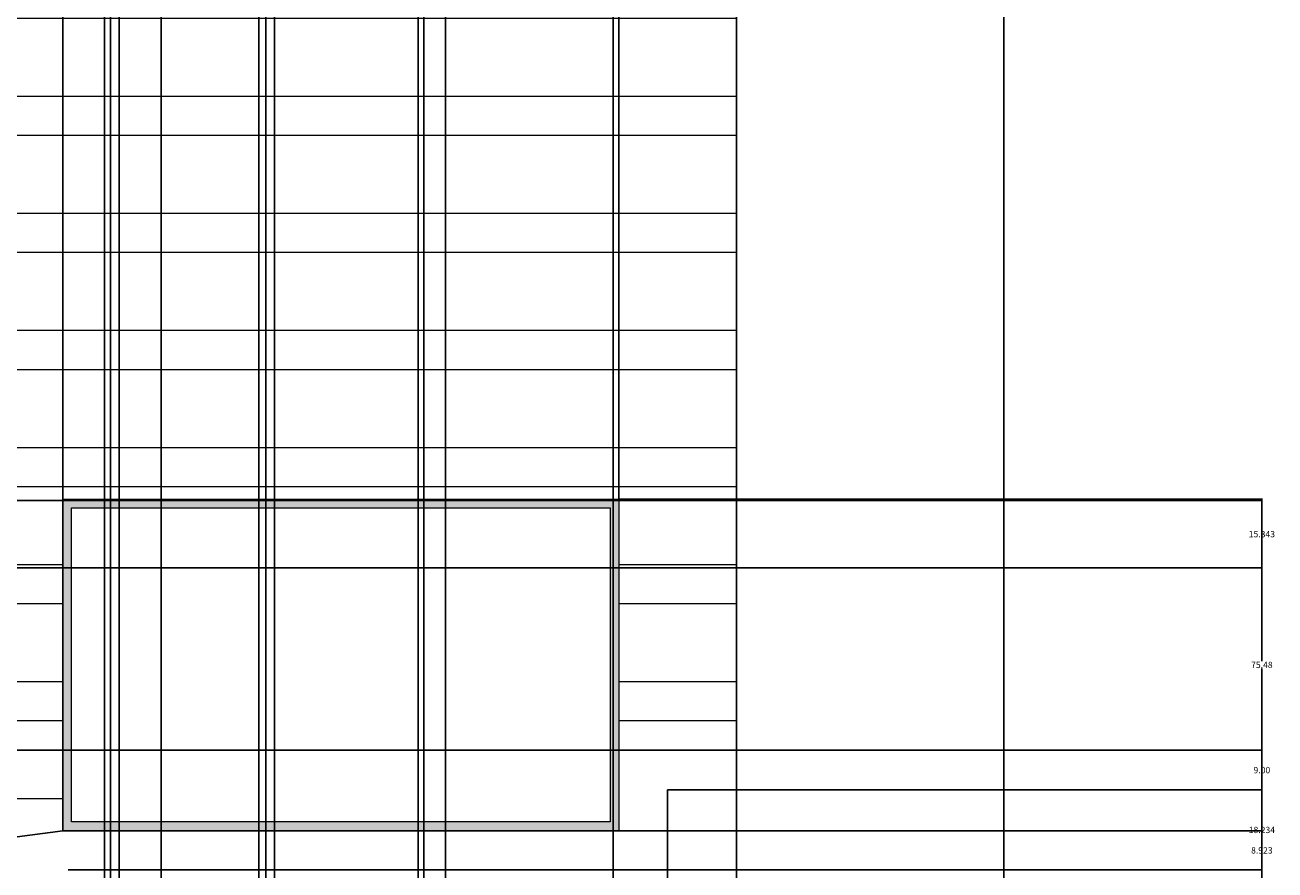
# Model space of a CAD drawing. Units: inches. Extents: x 241 to 943, y 109 to 1396.
# Tile 5 of 34: x 659 to 943, y 206 to 398. Entities that reach past the tile are written whole.
import ezdxf

# ---------------------------------------------------------------- set-up
doc = ezdxf.new("R2010")
doc.units = ezdxf.units.IN
doc.header["$MEASUREMENT"] = 0
for name, color, linetype, lineweight in [('A-ANNO-DIMS', 2, 'Continuous', 18), ('A-ELEV', 7, 'Continuous', 25), ('A-ELEV-SHAD', 9, 'Continuous', 13), ('A-GLAZ', 4, 'Continuous', 18), ('A-GLAZ-PATT', 18, 'Continuous', 13), ('A-WALL-PATT', 8, 'Continuous', 13)]:
    doc.layers.add(name, color=color, linetype=linetype, lineweight=lineweight)
doc.styles.get("Standard").update_dxf_attribs({"font": 'arial.ttf'})
doc.dimstyles.get("Standard").update_dxf_attribs({"dimtxt": 1.4375, "dimasz": 0.18, "dimexe": 0.18, "dimexo": 0.0625, "dimgap": 0.09, "dimtad": 0, "dimtih": 1, "dimtoh": 1, "dimdec": 4, "dimzin": 0, "dimdsep": 46, "dimlunit": 4, "dimtxsty": 'Standard', "dimcen": 0.09, "dimadec": 0, "dimazin": 0, "dimtfac": 1, "dimtdec": 4, "dimtofl": 0, "dimtmove": 0, "dimatfit": 3, "dimfxl": 1, "dimtolj": 1, "dimtzin": 0, "dimarcsym": 0})

# ---------------------------------------------------------------- blocks, each defined once
blk = doc.blocks.new('*D4')
at = {"layer": 'A-ANNO-DIMS', "color": 0, "lineweight": -2, "transparency": 16777216}
for p, q in [((820.84, 232.77), (820.84, 109.81)), ((377.04, 177.64), (377.04, 109.81)), ((377.22, 109.99), (596.39, 109.99)), ((820.66, 109.99), (601.48, 109.99))]:
    blk.add_line(p, q, dxfattribs=at)
at = {"layer": 'A-ANNO-DIMS', "color": 0, "transparency": 16777216}
for points in [[(377.22, 110.02), (377.22, 109.96), (377.04, 109.99)], [(820.66, 110.02), (820.66, 109.96), (820.84, 109.99)]]:
    blk.add_solid(points, dxfattribs=at)
at = {"layer": 'Defpoints', "color": 0, "transparency": 16777216}
for p in [(820.84, 232.83), (377.04, 177.7), (820.84, 109.99)]:
    blk.add_point(p, dxfattribs=at)
at = {"layer": 'A-ANNO-DIMS', "color": 0, "transparency": 16777216, "insert": (598.94, 109.99), "char_height": 1.438, "attachment_point": 5}
blk.add_mtext('\\A1;443.8', dxfattribs=at)
blk = doc.blocks.new('*D6')
at = {"layer": 'A-ANNO-DIMS', "color": 0, "lineweight": -2, "transparency": 16777216}
for p, q in [((820.84, 232.89), (820.84, 1395.05)), ((821.02, 1394.87), (848.73, 1394.87)), ((881.49, 1394.87), (853.77, 1394.87)), ((881.67, 232.89), (881.67, 1395.05))]:
    blk.add_line(p, q, dxfattribs=at)
at = {"layer": 'A-ANNO-DIMS', "color": 0, "transparency": 16777216}
for points in [[(821.02, 1394.9), (821.02, 1394.84), (820.84, 1394.87)], [(881.49, 1394.9), (881.49, 1394.84), (881.67, 1394.87)]]:
    blk.add_solid(points, dxfattribs=at)
at = {"layer": 'Defpoints', "color": 0, "transparency": 16777216}
for p in [(881.67, 1394.87), (820.84, 232.83), (881.67, 232.83)]:
    blk.add_point(p, dxfattribs=at)
at = {"layer": 'A-ANNO-DIMS', "color": 0, "transparency": 16777216, "insert": (851.25, 1394.87), "char_height": 1.438, "attachment_point": 5}
blk.add_mtext('\\A1;60.83', dxfattribs=at)
blk = doc.blocks.new('*D13')
at = {"layer": 'A-ANNO-DIMS', "color": 0, "lineweight": -2, "transparency": 16777216}
for p, q in [((650.91, 384.24), (650.91, 1395.05)), ((651.09, 1394.87), (656.14, 1394.87)), ((667.21, 1394.87), (662.16, 1394.87)), ((667.39, 290.06), (667.39, 1395.05))]:
    blk.add_line(p, q, dxfattribs=at)
at = {"layer": 'A-ANNO-DIMS', "color": 0, "transparency": 16777216}
for points in [[(651.09, 1394.9), (651.09, 1394.84), (650.91, 1394.87)], [(667.21, 1394.9), (667.21, 1394.84), (667.39, 1394.87)]]:
    blk.add_solid(points, dxfattribs=at)
at = {"layer": 'Defpoints', "color": 0, "transparency": 16777216}
for p in [(667.39, 1394.87), (650.91, 384.18), (667.39, 290)]:
    blk.add_point(p, dxfattribs=at)
at = {"layer": 'A-ANNO-DIMS', "color": 0, "transparency": 16777216, "insert": (659.15, 1394.87), "char_height": 1.438, "attachment_point": 5}
blk.add_mtext('\\A1;16.486', dxfattribs=at)
blk = doc.blocks.new('*D14')
at = {"layer": 'A-ANNO-DIMS', "color": 0, "lineweight": -2, "transparency": 16777216}
for p, q in [((667.39, 290.06), (667.39, 1395.05)), ((667.57, 1394.87), (727.7, 1394.87)), ((793.85, 1394.87), (733.72, 1394.87)), ((794.03, 290.06), (794.03, 1395.05))]:
    blk.add_line(p, q, dxfattribs=at)
at = {"layer": 'A-ANNO-DIMS', "color": 0, "transparency": 16777216}
for points in [[(667.57, 1394.9), (667.57, 1394.84), (667.39, 1394.87)], [(793.85, 1394.9), (793.85, 1394.84), (794.03, 1394.87)]]:
    blk.add_solid(points, dxfattribs=at)
at = {"layer": 'Defpoints', "color": 0, "transparency": 16777216}
for p in [(794.03, 1394.87), (667.39, 290), (794.03, 290)]:
    blk.add_point(p, dxfattribs=at)
at = {"layer": 'A-ANNO-DIMS', "color": 0, "transparency": 16777216, "insert": (730.71, 1394.87), "char_height": 1.438, "attachment_point": 5}
blk.add_mtext('\\A1;126.63', dxfattribs=at)
blk = doc.blocks.new('*D15')
at = {"layer": 'A-ANNO-DIMS', "color": 0, "lineweight": -2, "transparency": 16777216}
for p, q in [((794.03, 290.06), (794.03, 1395.05)), ((794.21, 1394.87), (805.04, 1394.87)), ((820.66, 1394.87), (809.82, 1394.87)), ((820.84, 232.89), (820.84, 1395.05))]:
    blk.add_line(p, q, dxfattribs=at)
at = {"layer": 'A-ANNO-DIMS', "color": 0, "transparency": 16777216}
for points in [[(794.21, 1394.9), (794.21, 1394.84), (794.03, 1394.87)], [(820.66, 1394.9), (820.66, 1394.84), (820.84, 1394.87)]]:
    blk.add_solid(points, dxfattribs=at)
at = {"layer": 'Defpoints', "color": 0, "transparency": 16777216}
for p in [(820.84, 1394.87), (794.03, 290), (820.84, 232.83)]:
    blk.add_point(p, dxfattribs=at)
at = {"layer": 'A-ANNO-DIMS', "color": 0, "transparency": 16777216, "insert": (807.43, 1394.87), "char_height": 1.438, "attachment_point": 5}
blk.add_mtext('\\A1;26.81', dxfattribs=at)
blk = doc.blocks.new('*D29')
at = {"layer": 'A-ANNO-DIMS', "color": 0, "lineweight": -2, "transparency": 16777216}
for p, q in [((462.17, 289.69), (940.6, 289.69)), ((940.42, 289.51), (940.42, 282.85)), ((940.42, 274.53), (940.42, 281.2)), ((462.17, 274.35), (940.6, 274.35))]:
    blk.add_line(p, q, dxfattribs=at)
at = {"layer": 'A-ANNO-DIMS', "color": 0, "transparency": 16777216}
for points in [[(940.39, 289.51), (940.45, 289.51), (940.42, 289.69)], [(940.39, 274.53), (940.45, 274.53), (940.42, 274.35)]]:
    blk.add_solid(points, dxfattribs=at)
at = {"layer": 'Defpoints', "color": 0, "transparency": 16777216}
for p in [(462.11, 289.69), (940.42, 289.69), (462.11, 274.35)]:
    blk.add_point(p, dxfattribs=at)
at = {"layer": 'A-ANNO-DIMS', "color": 0, "transparency": 16777216, "insert": (940.42, 282.02), "char_height": 1.438, "attachment_point": 5}
blk.add_mtext('\\A1;15.343', dxfattribs=at)
blk = doc.blocks.new('*D41')
at = {"layer": 'A-ANNO-DIMS', "color": 0, "lineweight": -2, "transparency": 16777216}
for p, q in [((820.77, 400.83), (244.31, 400.83)), ((244.49, 400.65), (244.49, 317.65)), ((244.49, 233.01), (244.49, 316.01)), ((820.77, 232.83), (244.31, 232.83))]:
    blk.add_line(p, q, dxfattribs=at)
at = {"layer": 'A-ANNO-DIMS', "color": 0, "transparency": 16777216}
for points in [[(244.46, 400.65), (244.52, 400.65), (244.49, 400.83)], [(244.46, 233.01), (244.52, 233.01), (244.49, 232.83)]]:
    blk.add_solid(points, dxfattribs=at)
at = {"layer": 'Defpoints', "color": 0, "transparency": 16777216}
for p in [(244.49, 400.83), (820.84, 400.83), (820.84, 232.83)]:
    blk.add_point(p, dxfattribs=at)
at = {"layer": 'A-ANNO-DIMS', "color": 0, "transparency": 16777216, "insert": (244.49, 316.83), "char_height": 1.438, "attachment_point": 5}
blk.add_mtext('\\A1;168', dxfattribs=at)
blk = doc.blocks.new('*D44')
at = {"layer": 'A-ANNO-DIMS', "color": 0, "lineweight": -2, "transparency": 16777216}
for p, q in [((794.09, 290), (940.6, 290)), ((940.42, 289.82), (940.42, 253.08)), ((940.42, 214.7), (940.42, 251.43)), ((794.09, 214.52), (940.6, 214.52))]:
    blk.add_line(p, q, dxfattribs=at)
at = {"layer": 'A-ANNO-DIMS', "color": 0, "transparency": 16777216}
for points in [[(940.39, 289.82), (940.45, 289.82), (940.42, 290)], [(940.39, 214.7), (940.45, 214.7), (940.42, 214.52)]]:
    blk.add_solid(points, dxfattribs=at)
at = {"layer": 'Defpoints', "color": 0, "transparency": 16777216}
for p in [(794.03, 290), (940.42, 290), (794.03, 214.52)]:
    blk.add_point(p, dxfattribs=at)
at = {"layer": 'A-ANNO-DIMS', "color": 0, "transparency": 16777216, "insert": (940.42, 252.26), "char_height": 1.438, "attachment_point": 5}
blk.add_mtext('\\A1;75.48', dxfattribs=at)
blk = doc.blocks.new('*D75')
at = {"layer": 'A-ANNO-DIMS', "color": 0, "lineweight": -2, "transparency": 16777216}
for p, q in [((667.46, 214.52), (940.6, 214.52)), ((940.42, 214.34), (940.42, 196.93)), ((940.42, 177.88), (940.42, 195.28)), ((377.1, 177.7), (940.6, 177.7))]:
    blk.add_line(p, q, dxfattribs=at)
at = {"layer": 'A-ANNO-DIMS', "color": 0, "transparency": 16777216}
for points in [[(940.39, 214.34), (940.45, 214.34), (940.42, 214.52)], [(940.39, 177.88), (940.45, 177.88), (940.42, 177.7)]]:
    blk.add_solid(points, dxfattribs=at)
at = {"layer": 'Defpoints', "color": 0, "transparency": 16777216}
for p in [(667.39, 214.52), (940.42, 214.52), (377.04, 177.7)]:
    blk.add_point(p, dxfattribs=at)
at = {"layer": 'A-ANNO-DIMS', "color": 0, "transparency": 16777216, "insert": (940.42, 196.11), "char_height": 1.438, "attachment_point": 5}
blk.add_mtext('\\A1;36.82', dxfattribs=at)
blk = doc.blocks.new('*D76')
at = {"layer": 'A-ANNO-DIMS', "color": 0, "lineweight": -2, "transparency": 16777216}
for p, q in [((805.12, 223.83), (940.6, 223.83)), ((940.42, 223.65), (940.42, 215.54)), ((940.42, 205.78), (940.42, 213.89)), ((805.12, 205.6), (940.6, 205.6))]:
    blk.add_line(p, q, dxfattribs=at)
at = {"layer": 'A-ANNO-DIMS', "color": 0, "transparency": 16777216}
for points in [[(940.39, 223.65), (940.45, 223.65), (940.42, 223.83)], [(940.39, 205.78), (940.45, 205.78), (940.42, 205.6)]]:
    blk.add_solid(points, dxfattribs=at)
at = {"layer": 'Defpoints', "color": 0, "transparency": 16777216}
for p in [(805.06, 223.83), (940.42, 223.83), (805.06, 205.6)]:
    blk.add_point(p, dxfattribs=at)
at = {"layer": 'A-ANNO-DIMS', "color": 0, "transparency": 16777216, "insert": (940.42, 214.71), "char_height": 1.438, "attachment_point": 5}
blk.add_mtext('\\A1;18.234', dxfattribs=at)
blk = doc.blocks.new('*D77')
at = {"layer": 'A-ANNO-DIMS', "color": 0, "lineweight": -2, "transparency": 16777216}
for p, q in [((805.06, 223.77), (805.06, 109.81)), ((881.67, 223.77), (881.67, 109.81)), ((805.24, 109.99), (840.99, 109.99)), ((881.49, 109.99), (845.73, 109.99))]:
    blk.add_line(p, q, dxfattribs=at)
at = {"layer": 'A-ANNO-DIMS', "color": 0, "transparency": 16777216}
for points in [[(805.24, 110.02), (805.24, 109.96), (805.06, 109.99)], [(881.49, 110.02), (881.49, 109.96), (881.67, 109.99)]]:
    blk.add_solid(points, dxfattribs=at)
at = {"layer": 'Defpoints', "color": 0, "transparency": 16777216}
for p in [(805.06, 223.83), (881.67, 223.83), (881.67, 109.99)]:
    blk.add_point(p, dxfattribs=at)
at = {"layer": 'A-ANNO-DIMS', "color": 0, "transparency": 16777216, "insert": (843.36, 109.99), "char_height": 1.438, "attachment_point": 5}
blk.add_mtext('\\A1;76.61', dxfattribs=at)
blk = doc.blocks.new('*D78')
at = {"layer": 'A-ANNO-DIMS', "color": 0, "lineweight": -2, "transparency": 16777216}
for p, q in [((881.73, 232.83), (940.6, 232.83)), ((940.42, 232.65), (940.42, 229.15)), ((940.42, 224.01), (940.42, 227.51)), ((881.73, 223.83), (940.6, 223.83))]:
    blk.add_line(p, q, dxfattribs=at)
at = {"layer": 'A-ANNO-DIMS', "color": 0, "transparency": 16777216}
for points in [[(940.39, 232.65), (940.45, 232.65), (940.42, 232.83)], [(940.39, 224.01), (940.45, 224.01), (940.42, 223.83)]]:
    blk.add_solid(points, dxfattribs=at)
at = {"layer": 'Defpoints', "color": 0, "transparency": 16777216}
for p in [(881.67, 232.83), (940.42, 232.83), (881.67, 223.83)]:
    blk.add_point(p, dxfattribs=at)
at = {"layer": 'A-ANNO-DIMS', "color": 0, "transparency": 16777216, "insert": (940.42, 228.33), "char_height": 1.438, "attachment_point": 5}
blk.add_mtext('\\A1;9.00', dxfattribs=at)
blk = doc.blocks.new('*D97')
at = {"layer": 'A-ANNO-DIMS', "color": 0, "lineweight": -2, "transparency": 16777216}
for p, q in [((881.67, 223.77), (881.67, 109.81)), ((303.24, 168.68), (303.24, 109.81)), ((303.42, 109.99), (589.38, 109.99)), ((881.49, 109.99), (595.53, 109.99))]:
    blk.add_line(p, q, dxfattribs=at)
at = {"layer": 'A-ANNO-DIMS', "color": 0, "transparency": 16777216}
for points in [[(303.42, 110.02), (303.42, 109.96), (303.24, 109.99)], [(881.49, 110.02), (881.49, 109.96), (881.67, 109.99)]]:
    blk.add_solid(points, dxfattribs=at)
at = {"layer": 'Defpoints', "color": 0, "transparency": 16777216}
for p in [(881.67, 223.83), (303.24, 168.74), (881.67, 109.99)]:
    blk.add_point(p, dxfattribs=at)
at = {"layer": 'A-ANNO-DIMS', "color": 0, "transparency": 16777216, "insert": (592.45, 109.99), "char_height": 1.438, "attachment_point": 5}
blk.add_mtext('\\A1;578.43', dxfattribs=at)
blk = doc.blocks.new('*D99')
at = {"layer": 'A-ANNO-DIMS', "color": 0, "lineweight": -2, "transparency": 16777216}
for p, q in [((417.09, 181.71), (417.09, 1395.05)), ((417.27, 1394.87), (539.16, 1394.87)), ((667.21, 1394.87), (545.33, 1394.87)), ((667.39, 214.58), (667.39, 1395.05))]:
    blk.add_line(p, q, dxfattribs=at)
at = {"layer": 'A-ANNO-DIMS', "color": 0, "transparency": 16777216}
for points in [[(417.27, 1394.9), (417.27, 1394.84), (417.09, 1394.87)], [(667.21, 1394.9), (667.21, 1394.84), (667.39, 1394.87)]]:
    blk.add_solid(points, dxfattribs=at)
at = {"layer": 'Defpoints', "color": 0, "transparency": 16777216}
for p in [(667.39, 1394.87), (667.39, 214.52), (417.09, 181.65)]:
    blk.add_point(p, dxfattribs=at)
at = {"layer": 'A-ANNO-DIMS', "color": 0, "transparency": 16777216, "insert": (542.24, 1394.87), "char_height": 1.438, "attachment_point": 5}
blk.add_mtext('\\A1;250.30', dxfattribs=at)
blk = doc.blocks.new('*D100')
at = {"layer": 'A-ANNO-DIMS', "color": 0, "lineweight": -2, "transparency": 16777216}
for p, q in [((667.46, 214.52), (940.6, 214.52)), ((940.42, 214.34), (940.42, 210.88)), ((940.42, 205.78), (940.42, 209.23)), ((668.63, 205.6), (940.6, 205.6))]:
    blk.add_line(p, q, dxfattribs=at)
at = {"layer": 'A-ANNO-DIMS', "color": 0, "transparency": 16777216}
for points in [[(940.39, 214.34), (940.45, 214.34), (940.42, 214.52)], [(940.39, 205.78), (940.45, 205.78), (940.42, 205.6)]]:
    blk.add_solid(points, dxfattribs=at)
at = {"layer": 'Defpoints', "color": 0, "transparency": 16777216}
for p in [(667.39, 214.52), (940.42, 214.52), (668.57, 205.6)]:
    blk.add_point(p, dxfattribs=at)
at = {"layer": 'A-ANNO-DIMS', "color": 0, "transparency": 16777216, "insert": (940.42, 210.06), "char_height": 1.438, "attachment_point": 5}
blk.add_mtext('\\A1;8.923', dxfattribs=at)
blk = doc.blocks.new('*D120')
at = {"layer": 'A-ANNO-DIMS', "color": 0, "lineweight": -2, "transparency": 16777216}
for p, q in [((642.92, 734.79), (642.92, 109.81)), ((678.27, 734.79), (678.27, 109.81)), ((643.1, 109.99), (658.07, 109.99)), ((678.09, 109.99), (663.11, 109.99))]:
    blk.add_line(p, q, dxfattribs=at)
at = {"layer": 'A-ANNO-DIMS', "color": 0, "transparency": 16777216}
for points in [[(643.1, 110.02), (643.1, 109.96), (642.92, 109.99)], [(678.09, 110.02), (678.09, 109.96), (678.27, 109.99)]]:
    blk.add_solid(points, dxfattribs=at)
at = {"layer": 'Defpoints', "color": 0, "transparency": 16777216}
for p in [(642.92, 734.85), (678.27, 734.85), (678.27, 109.99)]:
    blk.add_point(p, dxfattribs=at)
at = {"layer": 'A-ANNO-DIMS', "color": 0, "transparency": 16777216, "insert": (660.59, 109.99), "char_height": 1.438, "attachment_point": 5}
blk.add_mtext('\\A1;35.35', dxfattribs=at)
blk = doc.blocks.new('*D121')
at = {"layer": 'A-ANNO-DIMS', "color": 0, "lineweight": -2, "transparency": 16777216}
for p, q in [((680.27, 736.86), (680.27, 109.81)), ((713.62, 736.86), (713.62, 109.81)), ((680.45, 109.99), (693.87, 109.99)), ((713.44, 109.99), (700.02, 109.99))]:
    blk.add_line(p, q, dxfattribs=at)
at = {"layer": 'A-ANNO-DIMS', "color": 0, "transparency": 16777216}
for points in [[(680.45, 110.02), (680.45, 109.96), (680.27, 109.99)], [(713.44, 110.02), (713.44, 109.96), (713.62, 109.99)]]:
    blk.add_solid(points, dxfattribs=at)
at = {"layer": 'Defpoints', "color": 0, "transparency": 16777216}
for p in [(680.27, 736.92), (713.62, 736.92), (713.62, 109.99)]:
    blk.add_point(p, dxfattribs=at)
at = {"layer": 'A-ANNO-DIMS', "color": 0, "transparency": 16777216, "insert": (696.95, 109.99), "char_height": 1.438, "attachment_point": 5}
blk.add_mtext('\\A1;33.356', dxfattribs=at)
blk = doc.blocks.new('*D122')
at = {"layer": 'A-ANNO-DIMS', "color": 0, "lineweight": -2, "transparency": 16777216}
for p, q in [((715.62, 734.79), (715.62, 109.81)), ((754.54, 734.79), (754.54, 109.81)), ((715.8, 109.99), (732.7, 109.99)), ((754.36, 109.99), (737.46, 109.99))]:
    blk.add_line(p, q, dxfattribs=at)
at = {"layer": 'A-ANNO-DIMS', "color": 0, "transparency": 16777216}
for points in [[(715.8, 110.02), (715.8, 109.96), (715.62, 109.99)], [(754.36, 110.02), (754.36, 109.96), (754.54, 109.99)]]:
    blk.add_solid(points, dxfattribs=at)
at = {"layer": 'Defpoints', "color": 0, "transparency": 16777216}
for p in [(715.62, 734.85), (754.54, 734.85), (754.54, 109.99)]:
    blk.add_point(p, dxfattribs=at)
at = {"layer": 'A-ANNO-DIMS', "color": 0, "transparency": 16777216, "insert": (735.08, 109.99), "char_height": 1.438, "attachment_point": 5}
blk.add_mtext('\\A1;38.91', dxfattribs=at)
blk = doc.blocks.new('*D123')
at = {"layer": 'A-ANNO-DIMS', "color": 0, "lineweight": -2, "transparency": 16777216}
for p, q in [((754.54, 734.79), (754.54, 109.81)), ((792.69, 734.79), (792.69, 109.81)), ((754.72, 109.99), (771.09, 109.99)), ((792.51, 109.99), (776.13, 109.99))]:
    blk.add_line(p, q, dxfattribs=at)
at = {"layer": 'A-ANNO-DIMS', "color": 0, "transparency": 16777216}
for points in [[(754.72, 110.02), (754.72, 109.96), (754.54, 109.99)], [(792.51, 110.02), (792.51, 109.96), (792.69, 109.99)]]:
    blk.add_solid(points, dxfattribs=at)
at = {"layer": 'Defpoints', "color": 0, "transparency": 16777216}
for p in [(754.54, 734.85), (792.69, 734.85), (792.69, 109.99)]:
    blk.add_point(p, dxfattribs=at)
at = {"layer": 'A-ANNO-DIMS', "color": 0, "transparency": 16777216, "insert": (773.61, 109.99), "char_height": 1.438, "attachment_point": 5}
blk.add_mtext('\\A1;38.15', dxfattribs=at)
blk = doc.blocks.new('*D132')
at = {"layer": 'A-ANNO-DIMS', "color": 0, "lineweight": -2, "transparency": 16777216}
for p, q in [((617.76, 626.34), (617.76, 109.81)), ((676.87, 628.34), (676.87, 109.81)), ((617.94, 109.99), (644.94, 109.99)), ((676.69, 109.99), (649.69, 109.99))]:
    blk.add_line(p, q, dxfattribs=at)
at = {"layer": 'A-ANNO-DIMS', "color": 0, "transparency": 16777216}
for points in [[(617.94, 110.02), (617.94, 109.96), (617.76, 109.99)], [(676.69, 110.02), (676.69, 109.96), (676.87, 109.99)]]:
    blk.add_solid(points, dxfattribs=at)
at = {"layer": 'Defpoints', "color": 0, "transparency": 16777216}
for p in [(617.76, 626.4), (676.87, 628.4), (676.87, 109.99)]:
    blk.add_point(p, dxfattribs=at)
at = {"layer": 'A-ANNO-DIMS', "color": 0, "transparency": 16777216, "insert": (647.31, 109.99), "char_height": 1.438, "attachment_point": 5}
blk.add_mtext('\\A1;59.11', dxfattribs=at)
blk = doc.blocks.new('*D133')
at = {"layer": 'A-ANNO-DIMS', "color": 0, "lineweight": -2, "transparency": 16777216}
for p, q in [((676.87, 628.34), (676.87, 109.81)), ((712.02, 628.34), (712.02, 109.81)), ((677.05, 109.99), (691.92, 109.99)), ((711.84, 109.99), (696.96, 109.99))]:
    blk.add_line(p, q, dxfattribs=at)
at = {"layer": 'A-ANNO-DIMS', "color": 0, "transparency": 16777216}
for points in [[(677.05, 110.02), (677.05, 109.96), (676.87, 109.99)], [(711.84, 110.02), (711.84, 109.96), (712.02, 109.99)]]:
    blk.add_solid(points, dxfattribs=at)
at = {"layer": 'Defpoints', "color": 0, "transparency": 16777216}
for p in [(676.87, 628.4), (712.02, 628.4), (712.02, 109.99)]:
    blk.add_point(p, dxfattribs=at)
at = {"layer": 'A-ANNO-DIMS', "color": 0, "transparency": 16777216, "insert": (694.44, 109.99), "char_height": 1.438, "attachment_point": 5}
blk.add_mtext('\\A1;35.15', dxfattribs=at)
blk = doc.blocks.new('*D134')
at = {"layer": 'A-ANNO-DIMS', "color": 0, "lineweight": -2, "transparency": 16777216}
for p, q in [((712.02, 628.34), (712.02, 109.81)), ((749.63, 626.34), (749.63, 109.81)), ((712.2, 109.99), (727.75, 109.99)), ((749.45, 109.99), (733.9, 109.99))]:
    blk.add_line(p, q, dxfattribs=at)
at = {"layer": 'A-ANNO-DIMS', "color": 0, "transparency": 16777216}
for points in [[(712.2, 110.02), (712.2, 109.96), (712.02, 109.99)], [(749.45, 110.02), (749.45, 109.96), (749.63, 109.99)]]:
    blk.add_solid(points, dxfattribs=at)
at = {"layer": 'Defpoints', "color": 0, "transparency": 16777216}
for p in [(712.02, 628.4), (749.63, 626.4), (749.63, 109.99)]:
    blk.add_point(p, dxfattribs=at)
at = {"layer": 'A-ANNO-DIMS', "color": 0, "transparency": 16777216, "insert": (730.82, 109.99), "char_height": 1.438, "attachment_point": 5}
blk.add_mtext('\\A1;37.616', dxfattribs=at)
blk = doc.blocks.new('*D142')
at = {"layer": 'A-ANNO-DIMS', "color": 0, "lineweight": -2, "transparency": 16777216}
for p, q in [((689.79, 498.38), (689.79, 109.81)), ((651.6, 496.38), (651.6, 109.81)), ((651.78, 109.99), (668.18, 109.99)), ((689.61, 109.99), (673.21, 109.99))]:
    blk.add_line(p, q, dxfattribs=at)
at = {"layer": 'A-ANNO-DIMS', "color": 0, "transparency": 16777216}
for points in [[(651.78, 110.02), (651.78, 109.96), (651.6, 109.99)], [(689.61, 110.02), (689.61, 109.96), (689.79, 109.99)]]:
    blk.add_solid(points, dxfattribs=at)
at = {"layer": 'Defpoints', "color": 0, "transparency": 16777216}
for p in [(689.79, 498.44), (651.6, 496.44), (689.79, 109.99)]:
    blk.add_point(p, dxfattribs=at)
at = {"layer": 'A-ANNO-DIMS', "color": 0, "transparency": 16777216, "insert": (670.7, 109.99), "char_height": 1.438, "attachment_point": 5}
blk.add_mtext('\\A1;38.20', dxfattribs=at)
blk = doc.blocks.new('*D143')
at = {"layer": 'A-ANNO-DIMS', "color": 0, "lineweight": -2, "transparency": 16777216}
for p, q in [((689.79, 498.38), (689.79, 109.81)), ((748.33, 498.38), (748.33, 109.81)), ((689.97, 109.99), (716.55, 109.99)), ((748.15, 109.99), (721.58, 109.99))]:
    blk.add_line(p, q, dxfattribs=at)
at = {"layer": 'A-ANNO-DIMS', "color": 0, "transparency": 16777216}
for points in [[(689.97, 110.02), (689.97, 109.96), (689.79, 109.99)], [(748.15, 110.02), (748.15, 109.96), (748.33, 109.99)]]:
    blk.add_solid(points, dxfattribs=at)
at = {"layer": 'Defpoints', "color": 0, "transparency": 16777216}
for p in [(689.79, 498.44), (748.33, 498.44), (748.33, 109.99)]:
    blk.add_point(p, dxfattribs=at)
at = {"layer": 'A-ANNO-DIMS', "color": 0, "transparency": 16777216, "insert": (719.06, 109.99), "char_height": 1.438, "attachment_point": 5}
blk.add_mtext('\\A1;58.54', dxfattribs=at)
blk = doc.blocks.new('*D144')
at = {"layer": 'A-ANNO-DIMS', "color": 0, "lineweight": -2, "transparency": 16777216}
for p, q in [((748.33, 498.38), (748.33, 109.81)), ((792.69, 496.38), (792.69, 109.81)), ((748.51, 109.99), (767.97, 109.99)), ((792.51, 109.99), (773.06, 109.99))]:
    blk.add_line(p, q, dxfattribs=at)
at = {"layer": 'A-ANNO-DIMS', "color": 0, "transparency": 16777216}
for points in [[(748.51, 110.02), (748.51, 109.96), (748.33, 109.99)], [(792.51, 110.02), (792.51, 109.96), (792.69, 109.99)]]:
    blk.add_solid(points, dxfattribs=at)
at = {"layer": 'Defpoints', "color": 0, "transparency": 16777216}
for p in [(748.33, 498.44), (792.69, 496.44), (792.69, 109.99)]:
    blk.add_point(p, dxfattribs=at)
at = {"layer": 'A-ANNO-DIMS', "color": 0, "transparency": 16777216, "insert": (770.51, 109.99), "char_height": 1.438, "attachment_point": 5}
blk.add_mtext('\\A1;44.36', dxfattribs=at)

msp = doc.modelspace()

# ---------------------------------------------------------------- hatches: boundary and pattern name
at = {"layer": 'A-ELEV-SHAD'}
h = msp.add_hatch(color=256, dxfattribs=at)
h.dxf.hatch_style = 1
h.paths.add_polyline_path([(748.3325, 566.8295), (746.3325, 566.8295), (746.3325, 498.4395), (748.3325, 498.4395)])
h.paths.add_polyline_path([(746.3325, 524.3723), (691.794, 524.3723), (691.794, 522.3723), (746.3325, 522.3723)])
h.paths.add_polyline_path([(691.794, 566.8295), (689.794, 566.8295), (689.794, 498.4395), (691.794, 498.4395)])
h.paths.add_polyline_path([(790.691, 542.7994), (748.3325, 542.7994), (748.3325, 540.7994), (790.691, 540.7994)])
h.paths.add_polyline_path([(500.3323, 384.1784), (479.596, 384.1784), (479.596, 289.6933), (500.3323, 289.6933)])
h.paths.add_polyline_path([(481.596, 291.6933), (481.596, 382.1784), (498.3323, 382.1784), (498.3323, 291.6933)], flags=16)
h.paths.add_polyline_path([(462.1074, 384.1784), (390.895, 384.1784), (390.895, 289.6933), (462.1074, 289.6933)])
h.paths.add_polyline_path([(392.895, 291.6933), (392.895, 382.1784), (460.1074, 382.1784), (460.1074, 291.6933)], flags=16)
h.paths.add_polyline_path([(794.0275, 289.9984), (667.3935, 289.9984), (667.3935, 214.5189), (794.0275, 214.5189)])
h.paths.add_polyline_path([(792.0275, 287.9984), (792.0275, 216.5189), (669.3935, 216.5189), (669.3935, 287.9984)], flags=16)
h.paths.add_polyline_path([(508.0803, 525.3816), (506.0803, 525.3816), (506.0803, 521.3754), (452.9259, 521.3754), (452.9259, 525.3816), (450.9259, 525.3816), (450.9259, 519.3754), (508.0803, 519.3754)], flags=0)
h.paths.add_polyline_path([(508.0803, 566.8295), (450.9259, 566.8295), (450.9259, 527.3816), (452.9259, 527.3816), (452.9259, 564.8295), (506.0803, 564.8295), (506.0803, 527.3816), (508.0803, 527.3816)], flags=0)
h.paths.add_polyline_path([(537.4269, 566.8295), (534.1778, 566.8295), (534.1778, 527.3816), (537.4269, 527.3816)], flags=0)
h.paths.add_polyline_path([(537.4269, 525.3816), (534.1778, 525.3816), (534.1778, 508.9074), (537.4269, 508.9074)], flags=0)
h.paths.add_polyline_path([(565.2023, 568.8295), (424.1086, 568.8295), (424.1086, 496.4395), (565.2023, 496.4395)])
h.paths.add_polyline_path([(563.2023, 508.9074), (563.2023, 498.4395), (426.1086, 498.4395), (426.1086, 566.8295), (563.2023, 566.8295)], flags=16)
h.paths.add_polyline_path([(508.0803, 508.9074), (508.0803, 519.3754), (450.9259, 519.3754), (450.9259, 525.3816), (445.5808, 525.3816, -1), (445.5808, 527.3816), (450.9259, 527.3816), (450.9259, 566.8295), (508.0803, 566.8295), (537.4269, 566.8295), (537.4269, 508.9074)], flags=0)
h.paths.add_polyline_path([(506.0803, 521.3754), (452.9259, 521.3754), (452.9259, 564.8295), (506.0803, 564.8295)], flags=0)
at = {"layer": 'A-GLAZ-PATT'}
h = msp.add_hatch(dxfattribs=at)
h.set_pattern_fill('ANSI31', color=256, scale=34, angle=45)
h.paths.add_polyline_path([(486.3418, 786.9154), (413.1187, 786.9154), (413.1187, 761.2284), (486.3418, 761.2284)])
h.paths.add_polyline_path([(486.3418, 954.9154), (413.1187, 954.9154), (413.1187, 929.2284), (486.3418, 929.2284)])
h.paths.add_polyline_path([(462.1074, 289.6933), (390.895, 289.6933), (390.895, 277.4626), (390.895, 274.3507), (462.1074, 274.3507), (462.1074, 277.4626)])
h.paths.add_polyline_path([(500.3323, 289.6933), (479.596, 289.6933), (479.596, 274.3507), (500.3323, 274.3507)])
h.paths.add_polyline_path([(450.9259, 566.8295), (426.1086, 566.8295), (426.1086, 498.4395), (446.4348, 498.4395), (446.4348, 519.3754), (450.9259, 519.3754), (450.9259, 525.3816), (445.5808, 525.3816, -1), (445.5808, 527.3816), (450.9259, 527.3816)])
h.paths.add_polyline_path([(563.2023, 508.9074), (534.1778, 508.9074), (508.1906, 508.9074), (508.1906, 498.4395), (563.2023, 498.4395)])
h.paths.add_polyline_path([(747.6328, 700.7912), (712.0171, 700.7912), (712.0171, 628.4013), (747.6328, 628.4013)])
h.paths.add_polyline_path([(446.4348, 643.7483), (426.1086, 643.7483), (426.1086, 630.4013), (446.4348, 630.4013)])
h.paths.add_polyline_path([(564.8076, 841.5382), (553.5166, 841.5382), (508.3064, 841.5382), (508.3064, 782.5808), (564.8076, 782.5808)])
h.paths.add_polyline_path([(564.8076, 780.5808), (508.3064, 780.5808), (508.3064, 773.4916), (564.8076, 773.4916)])
h.paths.add_polyline_path([(792.691, 762.5799), (759.6248, 762.5799), (759.6248, 736.9235), (759.6248, 734.8538), (792.691, 734.8538)])
h.paths.add_polyline_path([(564.8076, 1009.5382), (553.5166, 1009.5382), (508.3064, 1009.5382), (508.3064, 950.5808), (562.3033, 950.5808, -1), (562.3033, 948.5808), (508.3064, 948.5808), (508.3064, 941.4916), (564.8076, 941.4916)])
h.paths.add_polyline_path([(486.3418, 1122.9154), (413.1187, 1122.9154), (413.1187, 1097.2284), (486.3418, 1097.2284)])
at = {"layer": 'A-WALL-PATT'}
h = msp.add_hatch(dxfattribs=at)
h.set_pattern_fill('ANSI32', color=256, scale=71, angle=135)
h.paths.add_polyline_path([(820.8374, 568.8295), (792.691, 568.8295), (792.691, 496.4395), (651.5974, 496.4395), (651.5974, 568.8295), (617.7594, 568.8295), (618.9643, 400.8295), (417.0913, 400.8295), (377.0391, 400.8295), (377.0391, 398.8538), (377.0391, 396.8782), (377.0391, 228.8782), (377.0391, 177.6977), (416.5078, 181.5724), (417.0913, 181.649), (530.2303, 196.5065), (530.2303, 384.1784), (650.907, 384.1784), (651.7861, 212.4693), (667.3935, 214.5189), (667.3935, 289.9984), (794.0275, 289.9984), (794.0275, 232.8295), (820.8374, 232.8295), (820.8374, 400.8295)])
h.paths.add_polyline_path([(500.3323, 384.1784), (500.3323, 289.6933), (500.3323, 274.3507), (479.596, 274.3507), (479.596, 289.6933), (479.596, 384.1784)], flags=16)
h.paths.add_polyline_path([(498.3323, 382.1784), (498.3323, 291.6933), (481.596, 291.6933), (481.596, 382.1784)], flags=0)
h.paths.add_polyline_path([(462.1074, 384.1784), (462.1074, 289.6933), (462.1074, 277.4626), (462.1074, 274.3507), (390.895, 274.3507), (390.895, 277.4626), (390.895, 289.6933), (390.895, 384.1784)], flags=16)
h.paths.add_polyline_path([(460.1074, 382.1784), (460.1074, 291.6933), (392.895, 291.6933), (392.895, 382.1784)], flags=0)
h.paths.add_polyline_path([(595.3136, 372.9401), (641.6196, 372.9401), (641.6196, 246.4081), (651.6121, 246.4593), (650.907, 384.1784), (530.2303, 384.1784), (530.2303, 245.8378), (595.3136, 246.1711)], flags=17)

# ---------------------------------------------------------------- linework, layer by layer
at = {"layer": 'A-ELEV'}
for p, q in [((820.8374, 400.8295), (820.8374, 232.8295)), ((820.8374, 232.8295), (794.0275, 232.8295)), ((820.8374, 232.8295), (881.5299, 232.8295)), ((881.5299, 232.8295), (881.667, 232.8295)), ((881.667, 223.8295), (881.667, 232.8295)), ((820.8374, 223.8295), (805.0568, 223.8295)), ((805.0568, 205.5955), (805.0568, 223.8295)), ((820.8374, 223.8295), (881.667, 223.8295)), ((667.3935, 214.5189), (417.0913, 181.649))]:
    msp.add_line(p, q, dxfattribs=at)
at = {"layer": 'A-GLAZ'}
for p, q in [((794.0275, 232.8295), (794.0275, 214.5189)), ((704.8945, 214.5189), (667.3935, 214.5189)), ((794.0275, 214.5189), (704.8945, 214.5189))]:
    msp.add_line(p, q, dxfattribs=at)
for points in [[(794.0275, 214.5189), (667.3935, 214.5189), (667.3935, 289.9984), (794.0275, 289.9984)], [(792.0275, 216.5189), (669.3935, 216.5189), (669.3935, 287.9984), (792.0275, 287.9984)]]:
    msp.add_lwpolyline(points, close=True, dxfattribs=at)

# ---------------------------------------------------------------- dimensions: what is measured, and where the dimension line sits
at = {"layer": 'A-ANNO-DIMS'}
for base, p1, p2, override, picture, middle in [((667.3935, 1394.8654), (417.0913, 181.649), (667.3935, 214.5189), {"dimdec": 2, "dimlfac": 1, "dimrnd": 0, "dimzin": 0, "dimdsep": 46, "dimlunit": 2}, '*D99', (542.2424, 1394.8654)), ((667.39345, 1394.86544), (650.90697, 384.17836), (667.39345, 289.99842), {"dimdec": 3, "dimlfac": 1, "dimrnd": 0, "dimzin": 0, "dimdsep": 46, "dimlunit": 2}, '*D13', (659.15021, 1394.86544)), ((794.0275, 1394.8654), (667.3935, 289.9984), (794.0275, 289.9984), {"dimdec": 2, "dimlfac": 1, "dimrnd": 0, "dimzin": 0, "dimdsep": 46, "dimlunit": 2}, '*D14', (730.7105, 1394.8654)), ((820.8374, 1394.8654), (794.0275, 289.9984), (820.8374, 232.8295), {"dimdec": 2, "dimlfac": 1, "dimrnd": 0, "dimzin": 0, "dimdsep": 46, "dimlunit": 2}, '*D15', (807.4324, 1394.8654)), ((881.667, 1394.8654), (820.8374, 232.8295), (881.667, 232.8295), {"dimdec": 2, "dimlfac": 1, "dimrnd": 0, "dimzin": 0, "dimdsep": 46, "dimlunit": 2}, '*D6', (851.2522, 1394.8654)), ((678.2674, 109.9907), (642.9197, 734.8538), (678.2674, 734.8538), {"dimdec": 2, "dimlfac": 1, "dimrnd": 0, "dimzin": 0, "dimdsep": 46, "dimlunit": 2}, '*D120', (660.5935, 109.9907)), ((713.6236, 109.9907), (680.2674, 736.9235), (713.6236, 736.9235), {"dimdec": 3, "dimlfac": 1, "dimrnd": 0, "dimzin": 0, "dimdsep": 46, "dimlunit": 2}, '*D121', (696.9455, 109.9907)), ((754.5373, 109.9907), (715.6236, 734.8538), (754.5373, 734.8538), {"dimdec": 2, "dimlfac": 1, "dimrnd": 0, "dimzin": 0, "dimdsep": 46, "dimlunit": 2}, '*D122', (735.0804, 109.9907)), ((792.691, 109.9907), (754.5373, 734.8538), (792.691, 734.8538), {"dimdec": 2, "dimlfac": 1, "dimrnd": 0, "dimzin": 0, "dimdsep": 46, "dimlunit": 2}, '*D123', (773.6142, 109.9907)), ((676.8698, 109.9907), (617.7594, 626.4013), (676.8698, 628.4013), {"dimdec": 2, "dimlfac": 1, "dimrnd": 0, "dimzin": 0, "dimdsep": 46, "dimlunit": 2}, '*D132', (647.3146, 109.9907)), ((712.0171, 109.9907), (676.8698, 628.4013), (712.0171, 628.4013), {"dimdec": 2, "dimlfac": 1, "dimrnd": 0, "dimzin": 0, "dimdsep": 46, "dimlunit": 2}, '*D133', (694.4435, 109.9907)), ((749.6328, 109.9907), (712.0171, 628.4013), (749.6328, 626.4013), {"dimdec": 3, "dimlfac": 1, "dimrnd": 0, "dimzin": 0, "dimdsep": 46, "dimlunit": 2}, '*D134', (730.825, 109.9907)), ((689.794, 109.9907), (651.5974, 496.4395), (689.794, 498.4395), {"dimdec": 2, "dimlfac": 1, "dimrnd": 0, "dimzin": 0, "dimdsep": 46, "dimlunit": 2}, '*D142', (670.6957, 109.9907)), ((748.3325, 109.9907), (689.794, 498.4395), (748.3325, 498.4395), {"dimdec": 2, "dimlfac": 1, "dimrnd": 0, "dimzin": 0, "dimdsep": 46, "dimlunit": 2}, '*D143', (719.0633, 109.9907)), ((792.691, 109.9907), (748.3325, 498.4395), (792.691, 496.4395), {"dimdec": 2, "dimlfac": 1, "dimrnd": 0, "dimzin": 0, "dimdsep": 46, "dimlunit": 2}, '*D144', (770.5118, 109.9907)), ((820.8374, 109.9907), (377.0391, 177.6977), (820.8374, 232.8295), {"dimdec": 1, "dimlfac": 1, "dimrnd": 0, "dimzin": 0, "dimdsep": 46, "dimlunit": 2}, '*D4', (598.9383, 109.9907)), ((881.667, 109.9907), (303.2358, 168.7407), (881.667, 223.8295), {"dimdec": 2, "dimlfac": 1, "dimrnd": 0, "dimzin": 0, "dimdsep": 46, "dimlunit": 2}, '*D97', (592.4514, 109.9907)), ((881.667, 109.9907), (805.0568, 223.8295), (881.667, 223.8295), {"dimdec": 2, "dimlfac": 1, "dimrnd": 0, "dimzin": 0, "dimdsep": 46, "dimlunit": 2}, '*D77', (843.3619, 109.9907))]:
    dim = msp.add_linear_dim(base=base, p1=p1, p2=p2, dimstyle='Standard', override=override, dxfattribs=at)
    dim.commit()
    dim.dimension.update_dxf_attribs({"geometry": picture, "text_midpoint": middle})
for base, p1, p2, override, picture, middle in [((244.4858, 400.8295), (820.8374, 232.8295), (820.8374, 400.8295), {"dimdec": 0, "dimlfac": 1, "dimrnd": 0, "dimzin": 0, "dimdsep": 46, "dimlunit": 2}, '*D41', (244.4858, 316.8295)), ((940.417, 289.6933), (462.1074, 274.3507), (462.1074, 289.6933), {"dimdec": 3, "dimlfac": 1, "dimrnd": 0, "dimzin": 0, "dimdsep": 46, "dimlunit": 2}, '*D29', (940.417, 282.022)), ((940.417, 289.9984), (794.0275, 214.5189), (794.0275, 289.9984), {"dimdec": 2, "dimlfac": 1, "dimrnd": 0, "dimzin": 0, "dimdsep": 46, "dimlunit": 2}, '*D44', (940.417, 252.2587)), ((940.417, 232.8295), (881.667, 223.8295), (881.667, 232.8295), {"dimdec": 2, "dimlfac": 1, "dimrnd": 0, "dimzin": 0, "dimdsep": 46, "dimlunit": 2}, '*D78', (940.417, 228.3295)), ((940.417, 223.8295), (805.0568, 205.5955), (805.0568, 223.8295), {"dimdec": 3, "dimlfac": 1, "dimrnd": 0, "dimzin": 0, "dimdsep": 46, "dimlunit": 2}, '*D76', (940.417, 214.7125)), ((940.417, 214.5189), (377.0391, 177.6977), (667.3935, 214.5189), {"dimdec": 2, "dimlfac": 1, "dimrnd": 0, "dimzin": 0, "dimdsep": 46, "dimlunit": 2}, '*D75', (940.417, 196.1083)), ((940.417, 214.5189), (668.5653, 205.5955), (667.3935, 214.5189), {"dimdec": 3, "dimlfac": 1, "dimrnd": 0, "dimzin": 0, "dimdsep": 46, "dimlunit": 2}, '*D100', (940.417, 210.0572))]:
    dim = msp.add_linear_dim(base=base, p1=p1, p2=p2, angle=90, dimstyle='Standard', override=override, dxfattribs=at)
    dim.commit()
    dim.dimension.update_dxf_attribs({"geometry": picture, "text_midpoint": middle})

doc.saveas('drawing.dxf')
